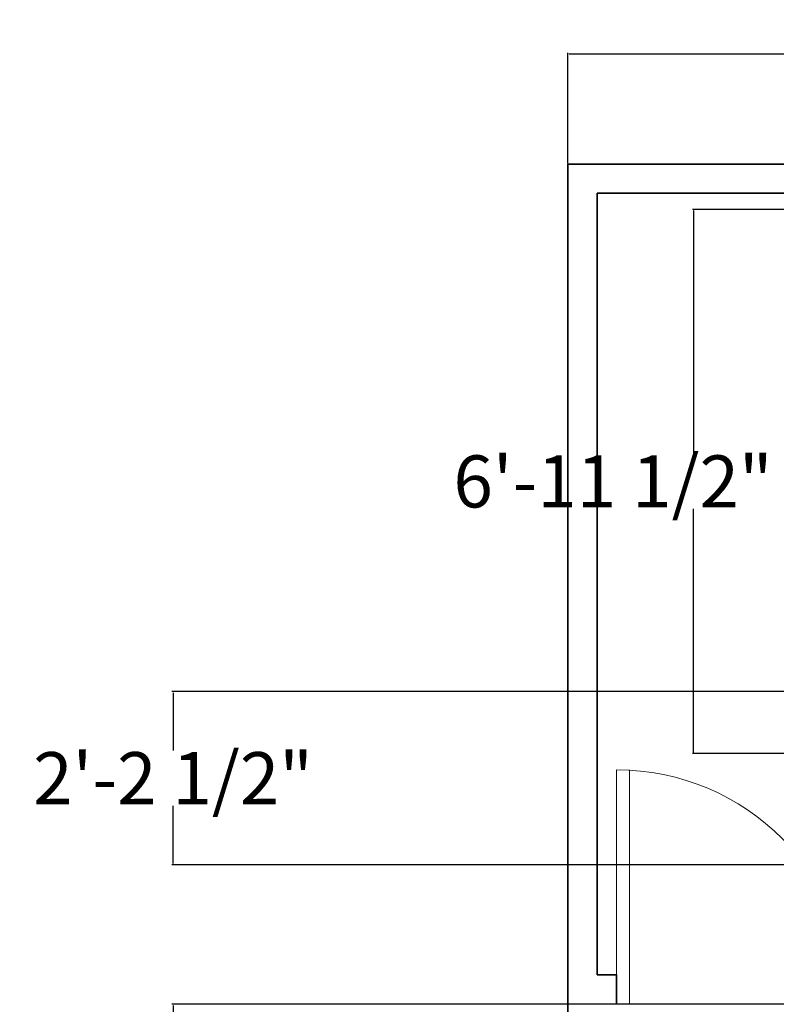
# Model space of a CAD drawing. Units: inches. Extents: x -438 to 102, y -60 to 1091.
# Tile 10 of 20: x -438 to -322, y 898 to 1049. Entities that reach past the tile are written whole.
import ezdxf

# ---------------------------------------------------------------- set-up
doc = ezdxf.new("R2010")
doc.units = ezdxf.units.IN
doc.header["$MEASUREMENT"] = 0
for name, color, linetype, lineweight, true_color in [('A-ANNO-DIMS', 217, 'Continuous', 18, 0x93278f), ('A-DOOR', 30, 'Continuous', 18, 0xf26722), ('A-WALL', 2, 'Continuous', 35, 0xf1eb1f), ('C-PROP', 2, 'Continuous', 35, 0xf1eb1f)]:
    doc.layers.add(name, color=color, linetype=linetype, lineweight=lineweight, true_color=true_color)
doc.styles.get("Standard").update_dxf_attribs({"font": 'arial.ttf'})
doc.dimstyles.get("Standard").update_dxf_attribs({"dimtxt": 8, "dimasz": 0.18, "dimexe": 0.18, "dimexo": 0.0625, "dimgap": 0.09, "dimtad": 0, "dimtih": 1, "dimtoh": 1, "dimdec": 4, "dimzin": 0, "dimdsep": 46, "dimlunit": 3, "dimtxsty": 'Standard', "dimcen": 0.09, "dimadec": 0, "dimazin": 0, "dimtfac": 1, "dimtdec": 4, "dimtofl": 0, "dimtmove": 0, "dimatfit": 3, "dimfxl": 1, "dimtolj": 1, "dimtzin": 0, "dimarcsym": 0})

# ---------------------------------------------------------------- blocks, each defined once
blk = doc.blocks.new('*D4')
at = {"layer": 'A-ANNO-DIMS', "color": 0, "lineweight": -2, "transparency": 16777216}
for p, q in [((-354.15, 1027.06), (-354.15, 1044.09)), ((-353.97, 1043.91), (-193.57, 1043.91)), ((28.67, 1043.91), (-131.73, 1043.91)), ((28.85, 1027.06), (28.85, 1044.09))]:
    blk.add_line(p, q, dxfattribs=at)
at = {"layer": 'A-ANNO-DIMS', "color": 0, "transparency": 16777216}
for points in [[(-353.97, 1043.94), (-353.97, 1043.88), (-354.15, 1043.91)], [(28.67, 1043.94), (28.67, 1043.88), (28.85, 1043.91)]]:
    blk.add_solid(points, dxfattribs=at)
at = {"layer": 'Defpoints', "color": 0, "transparency": 16777216}
for p in [(28.85, 1043.91), (-354.15, 1027), (28.85, 1027)]:
    blk.add_point(p, dxfattribs=at)
at = {"layer": 'A-ANNO-DIMS', "color": 0, "transparency": 16777216, "insert": (-162.65, 1043.91), "char_height": 8, "attachment_point": 5}
blk.add_mtext('\\A1;31\'-11.0000"', dxfattribs=at)
blk = doc.blocks.new('DOOR-SWING-36')
for p, q in [((-36, 0), (0, 0)), ((-2, 0), (-2, -36)), ((0, 0), (0, -36))]:
    blk.add_line(p, q)
blk.add_arc((0, 0), 36, 180, 270)
blk = doc.blocks.new('*D13')
at = {"layer": 'A-ANNO-DIMS', "color": 0, "lineweight": -2, "transparency": 16777216}
for p, q in [((-319.33, 1020.04), (-335.04, 1020.04)), ((-334.86, 1019.86), (-334.86, 982.5)), ((-334.86, 936.68), (-334.86, 974.04)), ((-319.33, 936.5), (-335.04, 936.5))]:
    blk.add_line(p, q, dxfattribs=at)
at = {"layer": 'A-ANNO-DIMS', "color": 0, "transparency": 16777216}
for points in [[(-334.89, 1019.86), (-334.83, 1019.86), (-334.86, 1020.04)], [(-334.89, 936.68), (-334.83, 936.68), (-334.86, 936.5)]]:
    blk.add_solid(points, dxfattribs=at)
at = {"layer": 'Defpoints', "color": 0, "transparency": 16777216}
for p in [(-334.86, 1020.04), (-319.27, 1020.04), (-319.27, 936.5)]:
    blk.add_point(p, dxfattribs=at)
at = {"layer": 'A-ANNO-DIMS', "color": 0, "transparency": 16777216, "insert": (-334.86, 978.27), "char_height": 8, "attachment_point": 5}
blk.add_mtext('\\A1;6\'-11 1/2" TYP.', dxfattribs=at)
blk = doc.blocks.new('*D44')
at = {"layer": 'A-ANNO-DIMS', "color": 0, "lineweight": -2, "transparency": 16777216}
for p, q in [((-64.71, 946), (-414.94, 946)), ((-414.76, 945.82), (-414.76, 936.94)), ((-414.76, 919.6), (-414.76, 928.48)), ((-64.71, 919.42), (-414.94, 919.42))]:
    blk.add_line(p, q, dxfattribs=at)
at = {"layer": 'A-ANNO-DIMS', "color": 0, "transparency": 16777216}
for points in [[(-414.79, 945.82), (-414.73, 945.82), (-414.76, 946)], [(-414.79, 919.6), (-414.73, 919.6), (-414.76, 919.42)]]:
    blk.add_solid(points, dxfattribs=at)
at = {"layer": 'Defpoints', "color": 0, "transparency": 16777216}
for p in [(-64.65, 946), (-414.76, 919.42), (-64.65, 919.42)]:
    blk.add_point(p, dxfattribs=at)
at = {"layer": 'A-ANNO-DIMS', "color": 0, "transparency": 16777216, "insert": (-414.76, 932.71), "char_height": 8, "attachment_point": 5}
blk.add_mtext('\\A1;2\'-2 1/2"', dxfattribs=at)
blk = doc.blocks.new('*D56')
at = {"layer": 'A-ANNO-DIMS', "color": 0, "lineweight": -2, "transparency": 16777216}
for p, q in [((-303.21, 898), (-414.94, 898)), ((-414.76, 897.82), (-414.76, 890.54)), ((-414.76, 874.8), (-414.76, 882.08)), ((-291.6, 874.62), (-414.94, 874.62))]:
    blk.add_line(p, q, dxfattribs=at)
at = {"layer": 'A-ANNO-DIMS', "color": 0, "transparency": 16777216}
for points in [[(-414.79, 897.82), (-414.73, 897.82), (-414.76, 898)], [(-414.79, 874.8), (-414.73, 874.8), (-414.76, 874.62)]]:
    blk.add_solid(points, dxfattribs=at)
at = {"layer": 'Defpoints', "color": 0, "transparency": 16777216}
for p in [(-414.76, 898), (-303.15, 898), (-291.54, 874.62)]:
    blk.add_point(p, dxfattribs=at)
at = {"layer": 'A-ANNO-DIMS', "color": 0, "transparency": 16777216, "insert": (-414.76, 886.31), "char_height": 8, "attachment_point": 5}
blk.add_mtext('\\A1;1\'-11 1/2"', dxfattribs=at)

msp = doc.modelspace()

# ---------------------------------------------------------------- linework, layer by layer
at = {"layer": 'A-WALL'}
for p, q in [((-349.64649, 1022.49939), (-349.64649, 902.49939)), ((-187.64649, 1022.49939), (-349.64649, 1022.49939)), ((-346.7047, 902.49939), (-349.64649, 902.49939)), ((-346.7047, 902.49939), (-346.7047, 897.99939))]:
    msp.add_line(p, q, dxfattribs=at)
at = {"layer": 'C-PROP'}
for p, q in [((28.85351, 1026.99939), (-354.14649, 1026.99939)), ((-354.14649, 1026.99939), (-354.14649, 3.99939))]:
    msp.add_line(p, q, dxfattribs=at)

# ---------------------------------------------------------------- block references
at = {"layer": 'A-DOOR', "rotation": 180}
msp.add_blockref('DOOR-SWING-36', (-346.7047, 897.99939), dxfattribs=at)

# ---------------------------------------------------------------- dimensions: what is measured, and where the dimension line sits
at = {"layer": 'A-ANNO-DIMS'}
dim = msp.add_linear_dim(base=(28.85351, 1043.90502), p1=(-354.14649, 1026.99939), p2=(28.85351, 1026.99939), dimstyle='Standard', override={"dimclrd": 0, "dimclre": 0, "dimclrt": 0}, dxfattribs=at)
dim.commit()
dim.dimension.update_dxf_attribs({"geometry": '*D4', "text_midpoint": (-162.64649, 1043.90502)})
dim = msp.add_linear_dim(base=(-334.86456, 1020.04286), p1=(-319.26918, 936.49708), p2=(-319.26918, 1020.04286), angle=90, text='<> TYP.', dimstyle='Standard', override={"dimdec": 1, "dimlfac": 1, "dimrnd": 0, "dimzin": 1, "dimdsep": 46, "dimlunit": 4, "dimfrac": 2}, dxfattribs=at)
dim.commit()
dim.dimension.update_dxf_attribs({"geometry": '*D13', "text_midpoint": (-334.86456, 978.26997)})
for base, p1, p2, picture, middle in [((-414.76009, 919.41905), (-64.64649, 945.99939), (-64.64649, 919.41905), '*D44', (-414.76009, 932.70922)), ((-414.76009, 897.99939), (-291.54025, 874.62295), (-303.14649, 897.99939), '*D56', (-414.76009, 886.31117))]:
    dim = msp.add_linear_dim(base=base, p1=p1, p2=p2, angle=90, dimstyle='Standard', override={"dimdec": 1, "dimlfac": 1, "dimrnd": 0, "dimzin": 1, "dimdsep": 46, "dimlunit": 4, "dimfrac": 2}, dxfattribs=at)
    dim.commit()
    dim.dimension.update_dxf_attribs({"geometry": picture, "text_midpoint": middle})

doc.saveas('drawing.dxf')
